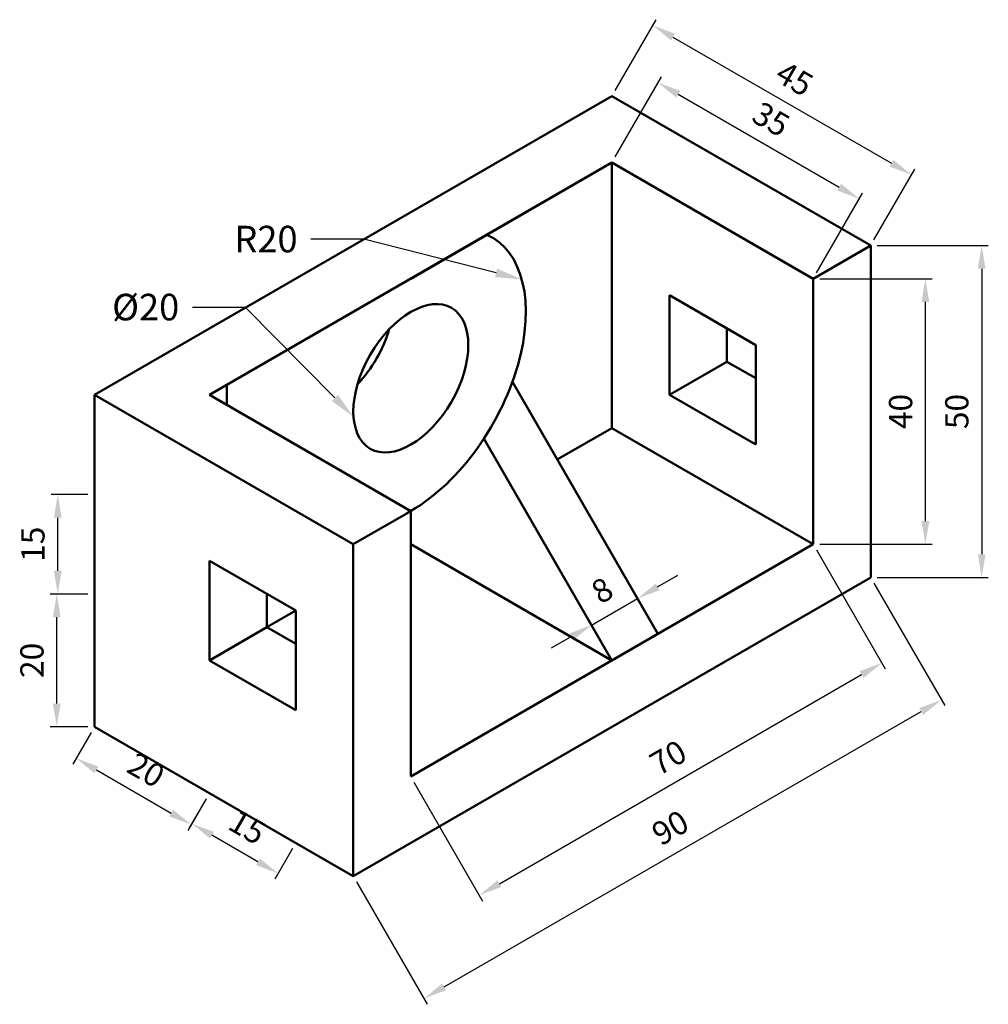
# Model space of a CAD drawing. Units: millimetres. Extents: x 1508 to 1654, y 1251 to 1399.
import ezdxf
from ezdxf import colors
from ezdxf.entities.mleader import LeaderData, LeaderLine
from ezdxf.math import Vec2, Vec3

# ---------------------------------------------------------------- set-up
doc = ezdxf.new("R2010")
doc.units = ezdxf.units.MM
for name, color, linetype, lineweight in [('M-DIMS', 3, 'Continuous', 25), ('M-OUTL', 7, 'Continuous', 50), ('M-TEXT', 7, 'Continuous', 25)]:
    doc.layers.add(name, color=color, linetype=linetype, lineweight=lineweight)
doc.styles.get("Standard").update_dxf_attribs({"font": 'arial.ttf'})
doc.dimstyles.new('AM_ISO$0', dxfattribs={"dimtxt": 3.5, "dimasz": 3.5, "dimexe": 1, "dimexo": 1, "dimgap": 1.5, "dimtad": 1, "dimdsep": 46, "dimtxsty": 'Standard', "dimcen": 0, "dimclrd": 256, "dimclre": 256, "dimclrt": 2, "dimadec": 0, "dimazin": 2, "dimtp": 0.1, "dimtm": 0.1, "dimtfac": 0.71, "dimtdec": 3, "dimtmove": 0, "dimatfit": 3, "dimfxl": 1, "dimlwd": -1, "dimlwe": -1, "dimarcsym": 1})

# ---------------------------------------------------------------- blocks, each defined once
blk = doc.blocks.new('*D3')
at = {"layer": 'Defpoints', "color": 0, "transparency": 16777216}
for p in [(1635.91, 1315.44), (1646.57, 1296.99), (1557.97, 1270.44)]:
    blk.add_point(p, dxfattribs=at)
at = {"layer": 'M-DIMS', "color": 0, "linetype": 'ByBlock', "transparency": 16777216}
for p, q in [((1636.41, 1314.58), (1647.07, 1296.13)), ((1571.66, 1253.74), (1643.54, 1295.24)), ((1558.47, 1269.58), (1569.13, 1251.13))]:
    blk.add_line(p, q, dxfattribs=at)
at = {"layer": 'M-DIMS', "color": 0, "transparency": 16777216}
for points in [[(1643.25, 1295.75), (1643.83, 1294.74), (1646.57, 1296.99)], [(1571.37, 1254.25), (1571.95, 1253.24), (1568.63, 1251.99)]]:
    blk.add_solid(points, dxfattribs=at)
at = {"layer": 'M-DIMS', "color": 0, "transparency": 16777216, "insert": (1605.95, 1277.34), "char_height": 3.5, "attachment_point": 5, "rotation": 30}
blk.add_mtext('90', dxfattribs=at)
blk = doc.blocks.new('*D4')
at = {"layer": 'Defpoints', "color": 0, "transparency": 16777216}
for p in [(1627.25, 1320.44), (1637.58, 1302.55), (1566.63, 1285.44)]:
    blk.add_point(p, dxfattribs=at)
at = {"layer": 'M-DIMS', "color": 0, "linetype": 'ByBlock', "transparency": 16777216}
for p, q in [((1627.75, 1319.58), (1638.08, 1301.69)), ((1579.99, 1269.3), (1634.55, 1300.8)), ((1567.13, 1284.58), (1577.46, 1266.69))]:
    blk.add_line(p, q, dxfattribs=at)
at = {"layer": 'M-DIMS', "color": 0, "transparency": 16777216}
for points in [[(1634.26, 1301.31), (1634.85, 1300.3), (1637.58, 1302.55)], [(1579.7, 1269.81), (1580.29, 1268.8), (1576.96, 1267.55)]]:
    blk.add_solid(points, dxfattribs=at)
at = {"layer": 'M-DIMS', "color": 0, "transparency": 16777216, "insert": (1605.63, 1287.9), "char_height": 3.5, "attachment_point": 5, "rotation": 30}
blk.add_mtext('70', dxfattribs=at)
blk = doc.blocks.new('*D5')
at = {"layer": 'Defpoints', "color": 0, "transparency": 16777216}
for p in [(1635.91, 1365.44), (1635.91, 1315.44), (1652.63, 1315.44)]:
    blk.add_point(p, dxfattribs=at)
at = {"layer": 'M-DIMS', "color": 0, "linetype": 'ByBlock', "transparency": 16777216}
for p, q in [((1636.91, 1365.44), (1653.63, 1365.44)), ((1652.63, 1361.94), (1652.63, 1318.94)), ((1636.91, 1315.44), (1653.63, 1315.44))]:
    blk.add_line(p, q, dxfattribs=at)
at = {"layer": 'M-DIMS', "color": 0, "transparency": 16777216}
for points in [[(1652.05, 1361.94), (1653.21, 1361.94), (1652.63, 1365.44)], [(1652.05, 1318.94), (1653.21, 1318.94), (1652.63, 1315.44)]]:
    blk.add_solid(points, dxfattribs=at)
at = {"layer": 'M-DIMS', "color": 0, "transparency": 16777216, "insert": (1649.34, 1340.44), "char_height": 3.5, "attachment_point": 5, "rotation": 90}
blk.add_mtext('50', dxfattribs=at)
blk = doc.blocks.new('*D6')
at = {"layer": 'Defpoints', "color": 0, "transparency": 16777216}
for p in [(1627.25, 1360.44), (1644.15, 1360.44), (1627.25, 1320.44)]:
    blk.add_point(p, dxfattribs=at)
at = {"layer": 'M-DIMS', "color": 0, "linetype": 'ByBlock', "transparency": 16777216}
for p, q in [((1628.25, 1360.44), (1645.15, 1360.44)), ((1644.15, 1323.94), (1644.15, 1356.94)), ((1628.25, 1320.44), (1645.15, 1320.44))]:
    blk.add_line(p, q, dxfattribs=at)
at = {"layer": 'M-DIMS', "color": 0, "transparency": 16777216}
for points in [[(1643.57, 1356.94), (1644.74, 1356.94), (1644.15, 1360.44)], [(1643.57, 1323.94), (1644.74, 1323.94), (1644.15, 1320.44)]]:
    blk.add_solid(points, dxfattribs=at)
at = {"layer": 'M-DIMS', "color": 0, "transparency": 16777216, "insert": (1640.87, 1340.44), "char_height": 3.5, "attachment_point": 5, "rotation": 90}
blk.add_mtext('40', dxfattribs=at)
blk = doc.blocks.new('*D7')
at = {"layer": 'Defpoints', "color": 0, "transparency": 16777216}
for p in [(1600.8, 1312.27), (1603.87, 1306.94), (1596.94, 1302.94)]:
    blk.add_point(p, dxfattribs=at)
at = {"layer": 'M-DIMS', "color": 0, "linetype": 'ByBlock', "transparency": 16777216}
for p, q in [((1603.83, 1314.02), (1606.86, 1315.77)), ((1603.37, 1307.81), (1600.3, 1313.13)), ((1593.87, 1308.27), (1600.8, 1312.27)), ((1596.44, 1303.81), (1593.37, 1309.13)), ((1590.84, 1306.52), (1587.81, 1304.77))]:
    blk.add_line(p, q, dxfattribs=at)
at = {"layer": 'M-DIMS', "color": 0, "transparency": 16777216}
for points in [[(1603.54, 1314.52), (1604.12, 1313.51), (1600.8, 1312.27)], [(1590.55, 1307.02), (1591.13, 1306.01), (1593.87, 1308.27)]]:
    blk.add_solid(points, dxfattribs=at)
at = {"layer": 'M-DIMS', "color": 0, "transparency": 16777216, "insert": (1595.69, 1313.11), "char_height": 3.5, "attachment_point": 5, "rotation": 30}
blk.add_mtext('8', dxfattribs=at)
blk = doc.blocks.new('*D8')
at = {"layer": 'Defpoints', "color": 0, "transparency": 16777216}
for p in [(1519, 1292.94), (1536.32, 1282.94), (1533.58, 1278.19)]:
    blk.add_point(p, dxfattribs=at)
at = {"layer": 'M-DIMS', "color": 0, "linetype": 'ByBlock', "transparency": 16777216}
for p, q in [((1518.5, 1292.08), (1515.76, 1287.33)), ((1519.29, 1286.44), (1530.55, 1279.94)), ((1535.82, 1282.08), (1533.08, 1277.33))]:
    blk.add_line(p, q, dxfattribs=at)
at = {"layer": 'M-DIMS', "color": 0, "transparency": 16777216}
for points in [[(1519.58, 1286.95), (1519, 1285.94), (1516.26, 1288.19)], [(1530.84, 1280.45), (1530.26, 1279.44), (1533.58, 1278.19)]]:
    blk.add_solid(points, dxfattribs=at)
at = {"layer": 'M-DIMS', "color": 0, "transparency": 16777216, "insert": (1526.56, 1286.04), "char_height": 3.5, "attachment_point": 5, "rotation": 330}
blk.add_mtext('20', dxfattribs=at)
blk = doc.blocks.new('*D9')
at = {"layer": 'Defpoints', "color": 0, "transparency": 16777216}
for p in [(1536.32, 1282.94), (1533.67, 1278.35), (1549.31, 1275.44)]:
    blk.add_point(p, dxfattribs=at)
at = {"layer": 'M-DIMS', "color": 0, "linetype": 'ByBlock', "transparency": 16777216}
for p, q in [((1535.82, 1282.08), (1533.17, 1277.49)), ((1543.63, 1272.6), (1536.7, 1276.6)), ((1548.81, 1274.58), (1546.16, 1269.99))]:
    blk.add_line(p, q, dxfattribs=at)
at = {"layer": 'M-DIMS', "color": 0, "transparency": 16777216}
for points in [[(1536.99, 1277.11), (1536.41, 1276.1), (1533.67, 1278.35)], [(1543.92, 1273.11), (1543.34, 1272.1), (1546.66, 1270.85)]]:
    blk.add_solid(points, dxfattribs=at)
at = {"layer": 'M-DIMS', "color": 0, "transparency": 16777216, "insert": (1541.81, 1277.45), "char_height": 3.5, "attachment_point": 5, "rotation": 330}
blk.add_mtext('15', dxfattribs=at)
blk = doc.blocks.new('*D10')
at = {"layer": 'Defpoints', "color": 0, "transparency": 16777216}
for p in [(1513.33, 1312.94), (1519, 1312.94), (1519, 1292.94)]:
    blk.add_point(p, dxfattribs=at)
at = {"layer": 'M-DIMS', "color": 0, "linetype": 'ByBlock', "transparency": 16777216}
for p, q in [((1518, 1312.94), (1512.33, 1312.94)), ((1513.33, 1296.44), (1513.33, 1309.44)), ((1518, 1292.94), (1512.33, 1292.94))]:
    blk.add_line(p, q, dxfattribs=at)
at = {"layer": 'M-DIMS', "color": 0, "transparency": 16777216}
for points in [[(1512.74, 1309.44), (1513.91, 1309.44), (1513.33, 1312.94)], [(1512.74, 1296.44), (1513.91, 1296.44), (1513.33, 1292.94)]]:
    blk.add_solid(points, dxfattribs=at)
at = {"layer": 'M-DIMS', "color": 0, "transparency": 16777216, "insert": (1510.04, 1302.94), "char_height": 3.5, "attachment_point": 5, "rotation": 90}
blk.add_mtext('20', dxfattribs=at)
blk = doc.blocks.new('*D11')
at = {"layer": 'Defpoints', "color": 0, "transparency": 16777216}
for p in [(1513.48, 1327.94), (1519, 1327.94), (1519, 1312.94)]:
    blk.add_point(p, dxfattribs=at)
at = {"layer": 'M-DIMS', "color": 0, "linetype": 'ByBlock', "transparency": 16777216}
for p, q in [((1518, 1327.94), (1512.48, 1327.94)), ((1513.48, 1316.44), (1513.48, 1324.44)), ((1518, 1312.94), (1512.48, 1312.94))]:
    blk.add_line(p, q, dxfattribs=at)
at = {"layer": 'M-DIMS', "color": 0, "transparency": 16777216}
for points in [[(1512.89, 1324.44), (1514.06, 1324.44), (1513.48, 1327.94)], [(1512.89, 1316.44), (1514.06, 1316.44), (1513.48, 1312.94)]]:
    blk.add_solid(points, dxfattribs=at)
at = {"layer": 'M-DIMS', "color": 0, "transparency": 16777216, "insert": (1510.19, 1320.44), "char_height": 3.5, "attachment_point": 5, "rotation": 90}
blk.add_mtext('15', dxfattribs=at)
blk = doc.blocks.new('*D12')
at = {"layer": 'Defpoints', "color": 0, "transparency": 16777216}
for p in [(1596.94, 1387.94), (1642.07, 1376.1), (1635.91, 1365.44)]:
    blk.add_point(p, dxfattribs=at)
at = {"layer": 'M-DIMS', "color": 0, "linetype": 'ByBlock', "transparency": 16777216}
for p, q in [((1597.44, 1388.81), (1603.6, 1399.47)), ((1606.13, 1396.85), (1639.04, 1377.85)), ((1636.41, 1366.31), (1642.57, 1376.97))]:
    blk.add_line(p, q, dxfattribs=at)
at = {"layer": 'M-DIMS', "color": 0, "transparency": 16777216}
for points in [[(1606.42, 1397.36), (1605.84, 1396.35), (1603.1, 1398.6)], [(1639.33, 1378.36), (1638.75, 1377.35), (1642.07, 1376.1)]]:
    blk.add_solid(points, dxfattribs=at)
at = {"layer": 'M-DIMS', "color": 0, "transparency": 16777216, "insert": (1624.22, 1390.19), "char_height": 3.5, "attachment_point": 5, "rotation": 330}
blk.add_mtext('45', dxfattribs=at)
blk = doc.blocks.new('*D13')
at = {"layer": 'Defpoints', "color": 0, "transparency": 16777216}
for p in [(1596.94, 1377.94), (1634.2, 1372.48), (1627.25, 1360.44)]:
    blk.add_point(p, dxfattribs=at)
at = {"layer": 'M-DIMS', "color": 0, "linetype": 'ByBlock', "transparency": 16777216}
for p, q in [((1597.44, 1378.81), (1604.39, 1390.85)), ((1606.92, 1388.23), (1631.17, 1374.23)), ((1627.75, 1361.31), (1634.7, 1373.35))]:
    blk.add_line(p, q, dxfattribs=at)
at = {"layer": 'M-DIMS', "color": 0, "transparency": 16777216}
for points in [[(1607.22, 1388.74), (1606.63, 1387.73), (1603.89, 1389.98)], [(1631.47, 1374.74), (1630.88, 1373.73), (1634.2, 1372.48)]]:
    blk.add_solid(points, dxfattribs=at)
at = {"layer": 'M-DIMS', "color": 0, "transparency": 16777216, "insert": (1620.69, 1384.08), "char_height": 3.5, "attachment_point": 5, "rotation": 330}
blk.add_mtext('35', dxfattribs=at)

msp = doc.modelspace()

# ---------------------------------------------------------------- linework, layer by layer
at = {"layer": 'M-OUTL'}
for p, q in [((1519.002, 1342.945), (1596.944, 1387.945)), ((1596.944, 1387.945), (1635.915, 1365.445)), ((1596.944, 1377.945), (1536.322, 1342.945)), ((1596.944, 1377.945), (1566.633, 1360.445)), ((1596.944, 1377.945), (1627.255, 1360.445)), ((1596.944, 1377.945), (1596.944, 1337.945)), ((1627.255, 1360.445), (1635.915, 1365.445)), ((1635.915, 1365.445), (1635.915, 1315.445)), ((1627.255, 1320.445), (1627.255, 1360.445)), ((1618.594, 1350.445), (1605.604, 1357.945)), ((1605.604, 1357.945), (1605.604, 1342.945)), ((1614.264, 1352.945), (1614.264, 1347.945)), ((1618.594, 1335.445), (1618.594, 1350.445)), ((1614.264, 1347.945), (1605.604, 1342.945)), ((1614.264, 1347.945), (1618.594, 1345.445)), ((1538.92, 1344.445), (1538.92, 1341.445)), ((1603.872, 1306.945), (1581.954, 1344.907)), ((1519.002, 1292.945), (1519.002, 1342.945)), ((1519.002, 1342.945), (1557.973, 1320.445)), ((1566.633, 1325.445), (1536.322, 1342.945)), ((1605.604, 1342.945), (1618.594, 1335.445)), ((1596.944, 1337.945), (1588.717, 1333.195)), ((1627.255, 1320.445), (1596.944, 1337.945)), ((1596.944, 1302.945), (1577.656, 1336.352)), ((1557.973, 1320.445), (1566.633, 1325.445)), ((1566.633, 1325.445), (1566.633, 1285.445)), ((1566.633, 1325.445), (1566.633, 1325.433)), ((1557.973, 1270.445), (1557.973, 1320.445)), ((1566.653, 1320.456), (1566.633, 1320.445)), ((1566.633, 1285.445), (1627.255, 1320.445)), ((1566.633, 1320.445), (1596.944, 1302.945)), ((1566.653, 1320.456), (1566.653, 1320.433)), ((1549.312, 1310.445), (1536.322, 1317.945)), ((1536.322, 1317.945), (1536.322, 1302.945)), ((1557.973, 1270.445), (1635.915, 1315.445)), ((1544.982, 1312.945), (1544.982, 1307.945)), ((1544.982, 1307.945), (1549.313, 1310.445)), ((1549.312, 1295.445), (1549.312, 1310.445)), ((1536.322, 1302.945), (1544.982, 1307.945)), ((1544.982, 1307.945), (1536.322, 1302.945)), ((1544.982, 1307.945), (1549.312, 1305.445)), ((1596.944, 1302.945), (1603.872, 1306.945)), ((1536.322, 1302.945), (1549.312, 1295.445)), ((1557.973, 1270.445), (1519.002, 1292.945))]:
    msp.add_line(p, q, dxfattribs=at)
for centre, major_axis, start_param, end_param in [((1566.653, 1345.445), (-12.247, -21.213), 7.0344822, 9.4883213), ((1555.375, 1351.945), (6.124, 10.607), 4.3077353, 5.1170426)]:
    msp.add_ellipse(centre, major_axis=major_axis, ratio=0.5773503, start_param=start_param, end_param=end_param, dxfattribs=at)
msp.add_ellipse((1566.653, 1345.445), major_axis=(-6.124, -10.607), ratio=0.5773503, dxfattribs=at)

# ---------------------------------------------------------------- dimensions: what is measured, and where the dimension line sits
at = {"layer": 'M-DIMS'}
for base, p1, p2, angle, picture, middle in [((1642.068, 1376.102), (1596.944, 1387.945), (1635.915, 1365.445), 330, '*D12', (1622.583, 1387.352)), ((1634.205, 1372.482), (1596.944, 1377.945), (1627.255, 1360.445), 330, '*D13', (1619.049, 1381.232)), ((1652.629, 1315.445), (1635.915, 1365.445), (1635.915, 1315.445), 270, '*D5', (1652.629, 1340.445)), ((1644.152, 1360.445), (1627.255, 1320.445), (1627.255, 1360.445), 90, '*D6', (1644.152, 1340.445)), ((1513.328, 1312.945), (1519.002, 1292.945), (1519.002, 1312.945), 90, '*D10', (1513.328, 1302.945))]:
    dim = msp.add_linear_dim(base=base, p1=p1, p2=p2, angle=angle, dimstyle='AM_ISO$0', override={"dimclrd": 0, "dimclre": 0, "dimclrt": 0}, dxfattribs=at)
    dim.commit()
    dim.dimension.update_dxf_attribs({"geometry": picture, "text_midpoint": middle, "dimtype": 161})
for p1, p2, distance, override, picture, middle in [((1519.002, 1312.945), (1519.002, 1327.945), 5.524, {"dimclrd": 0, "dimclre": 0, "dimclrt": 0}, '*D11', (1510.19, 1320.445)), ((1566.633, 1285.445), (1627.255, 1320.445), -20.66, {"dimclrd": 0, "dimclre": 0, "dimclrt": 0}, '*D4', (1605.63, 1287.899)), ((1557.973, 1270.445), (1635.915, 1315.445), -21.307, {"dimpost": '', "dimclrd": 0, "dimclre": 0, "dimclrt": 0}, '*D3', (1605.954, 1277.339)), ((1596.944, 1302.945), (1603.872, 1306.945), 6.145, {"dimpost": '', "dimclrd": 0, "dimclre": 0, "dimclrt": 0}, '*D7', (1595.692, 1313.113)), ((1519.002, 1292.945), (1536.322, 1282.945), -5.485, {"dimpost": '', "dimclrd": 0, "dimclre": 0, "dimclrt": 0}, '*D8', (1526.563, 1286.041)), ((1549.312, 1275.445), (1536.322, 1282.945), 5.304, {"dimpost": '', "dimclrd": 0, "dimclre": 0, "dimclrt": 0}, '*D9', (1541.809, 1277.448))]:
    dim = msp.add_aligned_dim(p1=p1, p2=p2, distance=distance, dimstyle='AM_ISO$0', override=override, dxfattribs=at)
    dim.commit()
    dim.dimension.update_dxf_attribs({"geometry": picture, "text_midpoint": middle})

# ---------------------------------------------------------------- leaders
at = {"layer": 'M-TEXT'}
ml = msp.add_multileader_mtext('Standard', dxfattribs=at)
ml.set_content('{\\C2;R20}', color=256)
ml.set_leader_properties()
ml.build(insert=Vec2(0, 0))
ctx = ml.context
ctx.base_point, ctx.plane_origin = Vec3(1538.054, 1366.383), Vec3(1583.366, 1360.346)
ctx.text_align_type = 2
notes = []
notes.append((ctx, [(0, (1, 1, 0), (1559.598, 1366.383), (-1, 0), 8, [(0, [(1583.366, 1360.346)], 0, [])])]))
ctx.mtext.insert, ctx.mtext.alignment, ctx.mtext.flow_direction = Vec3(1549.598, 1368.417), 3, 5
ml = msp.add_multileader_mtext('Standard', dxfattribs=at)
ml.set_content('{\\C2;%%C20}', color=256)
ml.set_leader_properties()
ml.build(insert=Vec2(0, 0))
ctx = ml.context
ctx.base_point, ctx.plane_origin = Vec3(1519.701, 1356.089), Vec3(1558.022, 1339.64)
ctx.text_align_type = 2
notes.append((ctx, [(0, (1, 1, 0), (1541.769, 1356.089), (-1, 0), 8, [(0, [(1558.022, 1339.64)], 0, [])])]))
ctx.mtext.insert, ctx.mtext.alignment, ctx.mtext.flow_direction = Vec3(1531.769, 1358.17), 3, 5
for ctx, leaders in notes:
    for number, flags, end, landing, length, lines in leaders:
        leader = LeaderData()
        leader.index, (leader.has_last_leader_line, leader.has_dogleg_vector, leader.attachment_direction) = number, flags
        leader.last_leader_point, leader.dogleg_vector, leader.dogleg_length = Vec3(end), Vec3(landing), length
        for number, points, colour, breaks in lines:
            line = LeaderLine()
            line.index, line.vertices, line.color, line.breaks = number, Vec3.list(points), colors.encode_raw_color(colour), breaks
            leader.lines.append(line)
        ctx.leaders.append(leader)

doc.saveas('drawing.dxf')
